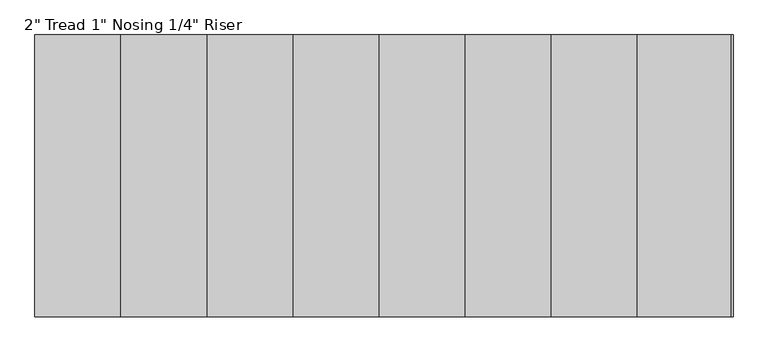
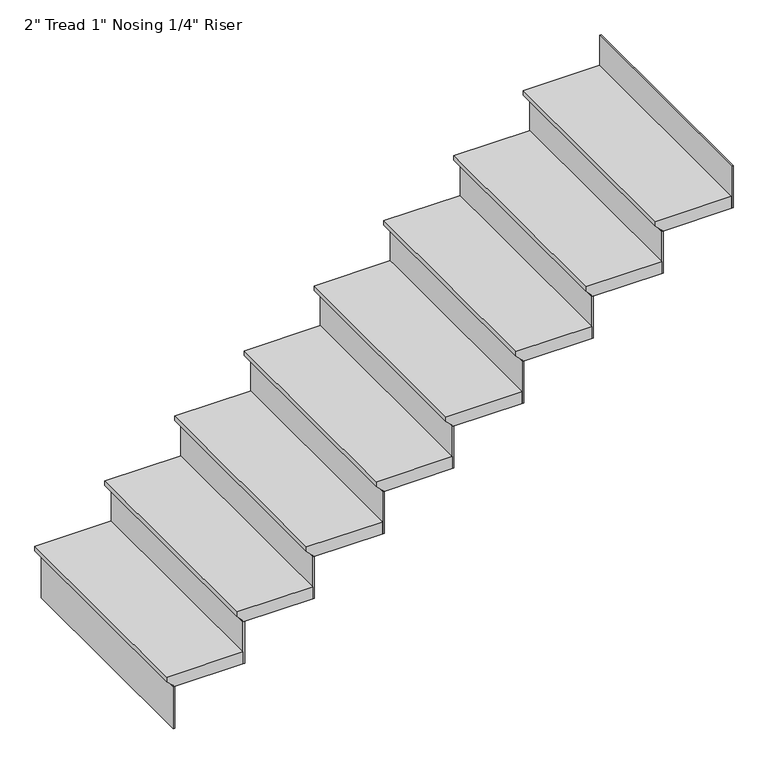
"""IFC4 building model written with IfcOpenShell, lengths in millimetres: stair flight geometry."""

from ifc_helpers import new_model, si_unit, frame, origin, place, context, project, spatial, polyline, outline, extrude, source, transform, mapped, element, save


def stair_flight_e53c0c70(model_context):
    return source(origin(), model_context, "Body", "SweptSolid", [
        extrude(outline(polyline([(4978.4, -6244.1591614), (4978.4, -6548.9591614), (4959.35, -6548.9591614), (4933.95, -6523.5591614), (4927.6, -6523.5591614), (4927.6, -6244.1591614), (4978.4, -6244.1591614)])), frame((0.0, 421.4825188, 0.0), z_axis=(0.0, 1.0, 0.0), x_axis=(0.0, 0.0, 1.0)), (0.0, 0.0, 1.0), 914.4),
        extrude(outline(polyline([(-6517.2091614, 421.4825188), (-6523.5591614, 421.4825188), (-6523.5591614, 1335.8825188), (-6517.2091614, 1335.8825188), (-6517.2091614, 421.4825188)])), frame((0.0, 0.0, 4749.8), z_axis=(0.0, 0.0, 1.0), x_axis=(1.0, 0.0, 0.0)), (0.0, 0.0, 1.0), 177.8),
        extrude(outline(polyline([(-6237.8091614, 421.4825188), (-6244.1591614, 421.4825188), (-6244.1591614, 1335.8825188), (-6237.8091614, 1335.8825188), (-6237.8091614, 421.4825188)])), frame((0.0, 0.0, 4927.6), z_axis=(0.0, 0.0, 1.0), x_axis=(1.0, 0.0, 0.0)), (0.0, 0.0, 1.0), 177.8),
        extrude(outline(polyline([(5156.2, -5964.7591614), (5156.2, -6269.5591614), (5137.15, -6269.5591614), (5111.75, -6244.1591614), (5105.4, -6244.1591614), (5105.4, -5964.7591614), (5156.2, -5964.7591614)])), frame((0.0, 421.4825188, 0.0), z_axis=(0.0, 1.0, 0.0), x_axis=(0.0, 0.0, 1.0)), (0.0, 0.0, 1.0), 914.4),
        extrude(outline(polyline([(-5958.4091614, 421.4825188), (-5964.7591614, 421.4825188), (-5964.7591614, 1335.8825188), (-5958.4091614, 1335.8825188), (-5958.4091614, 421.4825188)])), frame((0.0, 0.0, 5105.4), z_axis=(0.0, 0.0, 1.0), x_axis=(1.0, 0.0, 0.0)), (0.0, 0.0, 1.0), 177.8),
        extrude(outline(polyline([(5334.0, -5685.3591614), (5334.0, -5990.1591614), (5314.95, -5990.1591614), (5289.55, -5964.7591614), (5283.2, -5964.7591614), (5283.2, -5685.3591614), (5334.0, -5685.3591614)])), frame((0.0, 421.4825188, 0.0), z_axis=(0.0, 1.0, 0.0), x_axis=(0.0, 0.0, 1.0)), (0.0, 0.0, 1.0), 914.4),
        extrude(outline(polyline([(-5679.0091614, 421.4825188), (-5685.3591614, 421.4825188), (-5685.3591614, 1335.8825188), (-5679.0091614, 1335.8825188), (-5679.0091614, 421.4825188)])), frame((0.0, 0.0, 5283.2), z_axis=(0.0, 0.0, 1.0), x_axis=(1.0, 0.0, 0.0)), (0.0, 0.0, 1.0), 177.8),
        extrude(outline(polyline([(5511.8, -5405.9591614), (5511.8, -5710.7591614), (5492.75, -5710.7591614), (5467.35, -5685.3591614), (5461.0, -5685.3591614), (5461.0, -5405.9591614), (5511.8, -5405.9591614)])), frame((0.0, 421.4825188, 0.0), z_axis=(0.0, 1.0, 0.0), x_axis=(0.0, 0.0, 1.0)), (0.0, 0.0, 1.0), 914.4),
        extrude(outline(polyline([(-5399.6091614, 421.4825188), (-5405.9591614, 421.4825188), (-5405.9591614, 1335.8825188), (-5399.6091614, 1335.8825188), (-5399.6091614, 421.4825188)])), frame((0.0, 0.0, 5461.0), z_axis=(0.0, 0.0, 1.0), x_axis=(1.0, 0.0, 0.0)), (0.0, 0.0, 1.0), 177.8),
        extrude(outline(polyline([(5689.6, -5126.5591614), (5689.6, -5431.3591614), (5670.55, -5431.3591614), (5645.15, -5405.9591614), (5638.8, -5405.9591614), (5638.8, -5126.5591614), (5689.6, -5126.5591614)])), frame((0.0, 421.4825188, 0.0), z_axis=(0.0, 1.0, 0.0), x_axis=(0.0, 0.0, 1.0)), (0.0, 0.0, 1.0), 914.4),
        extrude(outline(polyline([(-5120.2091614, 421.4825188), (-5126.5591614, 421.4825188), (-5126.5591614, 1335.8825188), (-5120.2091614, 1335.8825188), (-5120.2091614, 421.4825188)])), frame((0.0, 0.0, 5638.8), z_axis=(0.0, 0.0, 1.0), x_axis=(1.0, 0.0, 0.0)), (0.0, 0.0, 1.0), 177.8),
        extrude(outline(polyline([(5867.4, -4847.1591614), (5867.4, -5151.9591614), (5848.35, -5151.9591614), (5822.95, -5126.5591614), (5816.6, -5126.5591614), (5816.6, -4847.1591614), (5867.4, -4847.1591614)])), frame((0.0, 421.4825188, 0.0), z_axis=(0.0, 1.0, 0.0), x_axis=(0.0, 0.0, 1.0)), (0.0, 0.0, 1.0), 914.4),
        extrude(outline(polyline([(-4840.8091614, 421.4825188), (-4847.1591614, 421.4825188), (-4847.1591614, 1335.8825188), (-4840.8091614, 1335.8825188), (-4840.8091614, 421.4825188)])), frame((0.0, 0.0, 5816.6), z_axis=(0.0, 0.0, 1.0), x_axis=(1.0, 0.0, 0.0)), (0.0, 0.0, 1.0), 177.8),
        extrude(outline(polyline([(6045.2, -4567.7591614), (6045.2, -4872.5591614), (6026.15, -4872.5591614), (6000.75, -4847.1591614), (5994.4, -4847.1591614), (5994.4, -4567.7591614), (6045.2, -4567.7591614)])), frame((0.0, 421.4825188, 0.0), z_axis=(0.0, 1.0, 0.0), x_axis=(0.0, 0.0, 1.0)), (0.0, 0.0, 1.0), 914.4),
        extrude(outline(polyline([(-4561.4091614, 421.4825188), (-4567.7591614, 421.4825188), (-4567.7591614, 1335.8825188), (-4561.4091614, 1335.8825188), (-4561.4091614, 421.4825188)])), frame((0.0, 0.0, 5994.4), z_axis=(0.0, 0.0, 1.0), x_axis=(1.0, 0.0, 0.0)), (0.0, 0.0, 1.0), 177.8),
        extrude(outline(polyline([(-4282.0091614, 421.4825188), (-4288.3591614, 421.4825188), (-4288.3591614, 1335.8825188), (-4282.0091614, 1335.8825188), (-4282.0091614, 421.4825188)])), frame((0.0, 0.0, 6172.2), z_axis=(0.0, 0.0, 1.0), x_axis=(1.0, 0.0, 0.0)), (0.0, 0.0, 1.0), 177.8),
        extrude(outline(polyline([(6223.0, -4288.3591614), (6223.0, -4593.1591614), (6203.95, -4593.1591614), (6178.55, -4567.7591614), (6172.2, -4567.7591614), (6172.2, -4288.3591614), (6223.0, -4288.3591614)])), frame((0.0, 421.4825188, 0.0), z_axis=(0.0, 1.0, 0.0), x_axis=(0.0, 0.0, 1.0)), (0.0, 0.0, 1.0), 914.4),
    ])


if __name__ == "__main__":
    model = new_model("IFC4")
    model_context = context("Model", 3, world=origin())
    ifc_project = project(units=[si_unit("LENGTHUNIT", "METRE", prefix="MILLI")], contexts=[model_context])
    site = spatial("IfcSite", under=ifc_project)
    building = spatial("IfcBuilding", under=site)
    placement = place(None, origin())
    stair_flight_shape = stair_flight_e53c0c70(model_context)
    element("IfcStairFlight", 1, ObjectType="2\" Tread 1\" Nosing 1/4\" Riser", at=placement, inside=building, context=model_context, shape_type="MappedRepresentation", body=[
        mapped(stair_flight_shape, transform((0.0, 0.0, 0.0), x_axis=(1.0, 0.0, 0.0), y_axis=(0.0, 1.0, 0.0), z_axis=(0.0, 0.0, 1.0))),
    ])
    save(model, "model.ifc")
